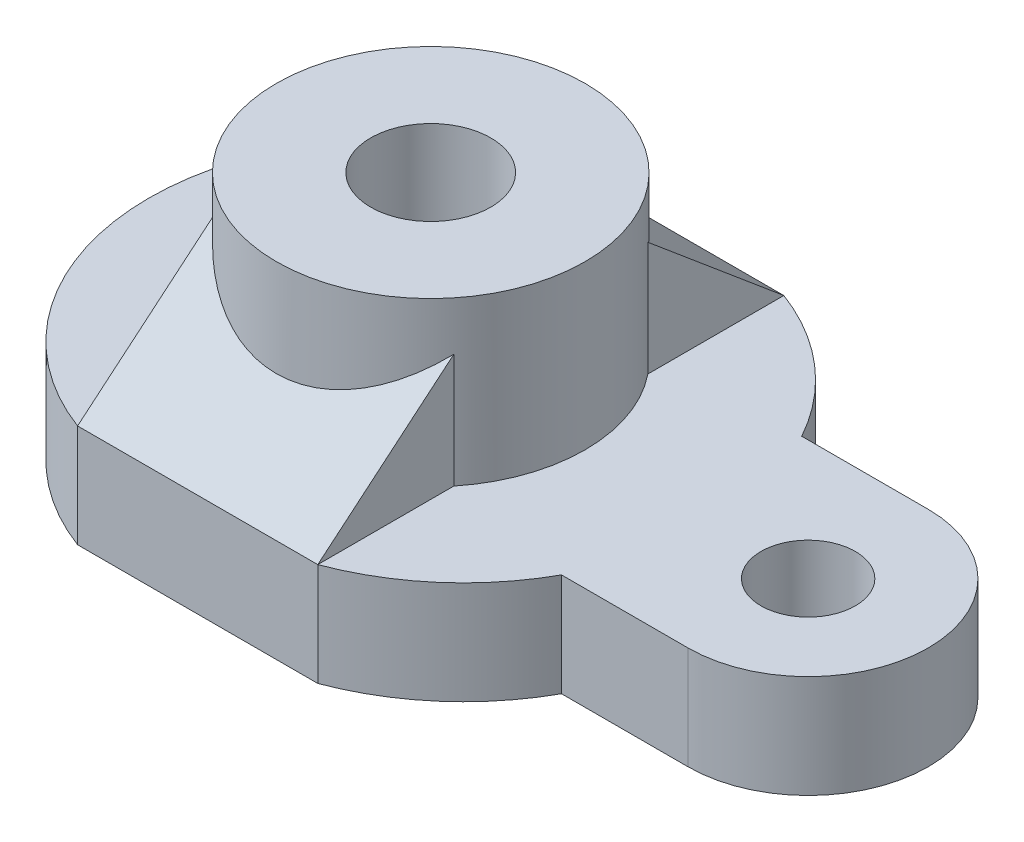
ISO-10303-21;
HEADER;
FILE_DESCRIPTION(('STEP AP214'),'2;1');
FILE_NAME('part.step','',(''),(''),'','','');
FILE_SCHEMA(('AUTOMOTIVE_DESIGN { 1 0 10303 214 1 1 1 1 }'));
ENDSEC;
DATA;
#1=APPLICATION_CONTEXT('core data for automotive mechanical design processes');
#2=APPLICATION_PROTOCOL_DEFINITION('international standard','automotive_design',2000,#1);
#3=PRODUCT_CONTEXT('',#1,'mechanical');
#4=PRODUCT('Part','Part','',(#3));
#5=PRODUCT_RELATED_PRODUCT_CATEGORY('part','',(#4));
#6=PRODUCT_DEFINITION_FORMATION('','',#4);
#7=PRODUCT_DEFINITION_CONTEXT('part definition',#1,'design');
#8=PRODUCT_DEFINITION('design','',#6,#7);
#9=PRODUCT_DEFINITION_SHAPE('','',#8);
#10=(LENGTH_UNIT() NAMED_UNIT(*) SI_UNIT(.MILLI.,.METRE.));
#11=(NAMED_UNIT(*) PLANE_ANGLE_UNIT() SI_UNIT($,.RADIAN.));
#12=(NAMED_UNIT(*) SI_UNIT($,.STERADIAN.) SOLID_ANGLE_UNIT());
#13=UNCERTAINTY_MEASURE_WITH_UNIT(LENGTH_MEASURE(1.E-05),#10,'distance_accuracy_value','');
#14=(GEOMETRIC_REPRESENTATION_CONTEXT(3) GLOBAL_UNCERTAINTY_ASSIGNED_CONTEXT((#13)) GLOBAL_UNIT_ASSIGNED_CONTEXT((#10,
#11,#12)) REPRESENTATION_CONTEXT('',''));
#15=CARTESIAN_POINT('',(0.,0.,0.));
#16=DIRECTION('',(0.,0.,1.));
#17=DIRECTION('',(1.,0.,0.));
#18=AXIS2_PLACEMENT_3D('',#15,#16,#17);
#19=CARTESIAN_POINT('',(-95.7034677287226,24.,0.));
#20=DIRECTION('',(0.,-1.,0.));
#21=DIRECTION('',(0.,0.,-1.));
#22=AXIS2_PLACEMENT_3D('',#19,#20,#21);
#23=PLANE('',#22);
#24=CARTESIAN_POINT('',(0.,24.,0.));
#25=DIRECTION('',(0.,1.,0.));
#26=DIRECTION('',(0.,0.,1.));
#27=AXIS2_PLACEMENT_3D('',#24,#25,#26);
#28=CIRCLE('',#27,11.);
#29=CARTESIAN_POINT('',(0.,24.,11.));
#30=VERTEX_POINT('',#29);
#31=EDGE_CURVE('E176',#30,#30,#28,.T.);
#32=ORIENTED_EDGE('',*,*,#31,.F.);
#33=EDGE_LOOP('',(#32));
#34=FACE_BOUND('',#33,.T.);
#35=DIRECTION('',(0.,0.,-1.));
#36=VECTOR('',#35,1.);
#37=CARTESIAN_POINT('',(-60.,24.,54.3327781156182));
#38=LINE('',#37,#36);
#39=CARTESIAN_POINT('',(-60.,24.,54.3327781156182));
#40=VERTEX_POINT('',#39);
#41=CARTESIAN_POINT('',(-60.,24.,22.6274169979695));
#42=VERTEX_POINT('',#41);
#43=EDGE_CURVE('E137',#40,#42,#38,.T.);
#44=ORIENTED_EDGE('',*,*,#43,.F.);
#45=CARTESIAN_POINT('',(-80.2965322712774,24.,0.));
#46=DIRECTION('',(0.,1.,0.));
#47=DIRECTION('',(0.,0.,-1.));
#48=AXIS2_PLACEMENT_3D('',#45,#46,#47);
#49=CIRCLE('',#48,58.);
#50=CARTESIAN_POINT('',(-29.5028318744762,24.,28.));
#51=VERTEX_POINT('',#50);
#52=EDGE_CURVE('E242',#40,#51,#49,.T.);
#53=ORIENTED_EDGE('',*,*,#52,.T.);
#54=DIRECTION('',(1.,0.,0.));
#55=VECTOR('',#54,1.);
#56=CARTESIAN_POINT('',(0.,24.,28.));
#57=LINE('',#56,#55);
#58=CARTESIAN_POINT('',(0.,24.,28.));
#59=VERTEX_POINT('',#58);
#60=EDGE_CURVE('E243',#51,#59,#57,.T.);
#61=ORIENTED_EDGE('',*,*,#60,.T.);
#62=CARTESIAN_POINT('',(0.,24.,0.));
#63=DIRECTION('',(0.,1.,0.));
#64=DIRECTION('',(0.,0.,1.));
#65=AXIS2_PLACEMENT_3D('',#62,#63,#64);
#66=CIRCLE('',#65,28.);
#67=CARTESIAN_POINT('',(0.,24.,-28.));
#68=VERTEX_POINT('',#67);
#69=EDGE_CURVE('E247',#59,#68,#66,.T.);
#70=ORIENTED_EDGE('',*,*,#69,.T.);
#71=DIRECTION('',(-1.,0.,0.));
#72=VECTOR('',#71,1.);
#73=CARTESIAN_POINT('',(0.,24.,-28.));
#74=LINE('',#73,#72);
#75=CARTESIAN_POINT('',(-29.5028318744762,24.,-28.));
#76=VERTEX_POINT('',#75);
#77=EDGE_CURVE('E155',#68,#76,#74,.T.);
#78=ORIENTED_EDGE('',*,*,#77,.T.);
#79=CARTESIAN_POINT('',(-80.2965322712774,24.,0.));
#80=DIRECTION('',(0.,1.,0.));
#81=DIRECTION('',(0.,0.,-1.));
#82=AXIS2_PLACEMENT_3D('',#79,#80,#81);
#83=CIRCLE('',#82,58.);
#84=CARTESIAN_POINT('',(-60.,24.,-54.3327781156181));
#85=VERTEX_POINT('',#84);
#86=EDGE_CURVE('E146',#76,#85,#83,.T.);
#87=ORIENTED_EDGE('',*,*,#86,.T.);
#88=CARTESIAN_POINT('',(-60.,24.,-22.6274169979695));
#89=VERTEX_POINT('',#88);
#90=EDGE_CURVE('E130',#89,#85,#38,.T.);
#91=ORIENTED_EDGE('',*,*,#90,.F.);
#92=CARTESIAN_POINT('',(-88.,24.,0.));
#93=DIRECTION('',(0.,1.,0.));
#94=DIRECTION('',(0.,0.,1.));
#95=AXIS2_PLACEMENT_3D('',#92,#93,#94);
#96=CIRCLE('',#95,36.);
#97=EDGE_CURVE('E212',#42,#89,#96,.T.);
#98=ORIENTED_EDGE('',*,*,#97,.F.);
#99=EDGE_LOOP('',(#44,#53,#61,#70,#78,#87,#91,#98));
#100=FACE_BOUND('',#99,.T.);
#101=ADVANCED_FACE('F39',(#34,#100),#23,.F.);
#102=CARTESIAN_POINT('',(-88.,62.,0.));
#103=DIRECTION('',(0.,-1.,0.));
#104=DIRECTION('',(0.,0.,-1.));
#105=AXIS2_PLACEMENT_3D('',#102,#103,#104);
#106=CYLINDRICAL_SURFACE('',#105,36.);
#107=CARTESIAN_POINT('',(-88.,62.,0.));
#108=DIRECTION('',(0.,1.,0.));
#109=DIRECTION('',(0.,0.,1.));
#110=AXIS2_PLACEMENT_3D('',#107,#108,#109);
#111=CIRCLE('',#110,36.);
#112=CARTESIAN_POINT('',(-88.,62.,36.));
#113=VERTEX_POINT('',#112);
#114=EDGE_CURVE('E232',#113,#113,#111,.T.);
#115=ORIENTED_EDGE('',*,*,#114,.F.);
#116=EDGE_LOOP('',(#115));
#117=FACE_BOUND('',#116,.T.);
#118=DIRECTION('',(0.,-1.,0.));
#119=VECTOR('',#118,1.);
#120=CARTESIAN_POINT('',(-60.,62.,-22.6274169979695));
#121=LINE('',#120,#119);
#122=CARTESIAN_POINT('',(-60.,50.6039568201611,-22.6274169979695));
#123=VERTEX_POINT('',#122);
#124=EDGE_CURVE('E11',#123,#89,#121,.T.);
#125=ORIENTED_EDGE('',*,*,#124,.F.);
#126=CARTESIAN_POINT('',(-88.,69.5906140776516,0.));
#127=DIRECTION('',(0.,-0.766044443118982,0.642787609686535));
#128=DIRECTION('',(0.,-0.642787609686535,-0.766044443118982));
#129=AXIS2_PLACEMENT_3D('',#126,#127,#128);
#130=ELLIPSE('',#129,46.9946624159618,36.);
#131=CARTESIAN_POINT('',(-116.,50.6039568201611,-22.6274169979695));
#132=VERTEX_POINT('',#131);
#133=EDGE_CURVE('E50',#132,#123,#130,.T.);
#134=ORIENTED_EDGE('',*,*,#133,.F.);
#135=DIRECTION('',(0.,-1.,0.));
#136=VECTOR('',#135,1.);
#137=CARTESIAN_POINT('',(-116.,62.,-22.6274169979695));
#138=LINE('',#137,#136);
#139=CARTESIAN_POINT('',(-116.,24.,-22.6274169979695));
#140=VERTEX_POINT('',#139);
#141=EDGE_CURVE('E217',#132,#140,#138,.T.);
#142=ORIENTED_EDGE('',*,*,#141,.T.);
#143=CARTESIAN_POINT('',(-116.,24.,22.6274169979695));
#144=VERTEX_POINT('',#143);
#145=EDGE_CURVE('E207',#140,#144,#96,.T.);
#146=ORIENTED_EDGE('',*,*,#145,.T.);
#147=DIRECTION('',(0.,-1.,0.));
#148=VECTOR('',#147,1.);
#149=CARTESIAN_POINT('',(-116.,62.,22.6274169979695));
#150=LINE('',#149,#148);
#151=CARTESIAN_POINT('',(-116.,50.6039568201612,22.6274169979695));
#152=VERTEX_POINT('',#151);
#153=EDGE_CURVE('E209',#144,#152,#150,.F.);
#154=ORIENTED_EDGE('',*,*,#153,.T.);
#155=CARTESIAN_POINT('',(-88.,69.5906140776517,0.));
#156=DIRECTION('',(0.,-0.766044443118982,-0.642787609686535));
#157=DIRECTION('',(0.,-0.642787609686535,0.766044443118982));
#158=AXIS2_PLACEMENT_3D('',#155,#156,#157);
#159=ELLIPSE('',#158,46.9946624159618,36.);
#160=CARTESIAN_POINT('',(-60.,50.6039568201612,22.6274169979695));
#161=VERTEX_POINT('',#160);
#162=EDGE_CURVE('E213',#161,#152,#159,.T.);
#163=ORIENTED_EDGE('',*,*,#162,.F.);
#164=DIRECTION('',(0.,-1.,0.));
#165=VECTOR('',#164,1.);
#166=CARTESIAN_POINT('',(-60.,62.,22.6274169979695));
#167=LINE('',#166,#165);
#168=EDGE_CURVE('E216',#42,#161,#167,.F.);
#169=ORIENTED_EDGE('',*,*,#168,.F.);
#170=ORIENTED_EDGE('',*,*,#97,.T.);
#171=EDGE_LOOP('',(#125,#134,#142,#146,#154,#163,#169,#170));
#172=FACE_BOUND('',#171,.T.);
#173=ADVANCED_FACE('F225',(#117,#172),#106,.T.);
#174=CARTESIAN_POINT('',(-95.7034677287226,24.,0.));
#175=DIRECTION('',(0.,1.,0.));
#176=DIRECTION('',(0.,0.,-1.));
#177=AXIS2_PLACEMENT_3D('',#174,#175,#176);
#178=CIRCLE('',#177,58.);
#179=CARTESIAN_POINT('',(-116.,24.,-54.3327781156181));
#180=VERTEX_POINT('',#179);
#181=CARTESIAN_POINT('',(-116.,24.,54.3327781156182));
#182=VERTEX_POINT('',#181);
#183=EDGE_CURVE('E192',#180,#182,#178,.T.);
#184=ORIENTED_EDGE('',*,*,#183,.T.);
#185=DIRECTION('',(0.,0.,-1.));
#186=VECTOR('',#185,1.);
#187=CARTESIAN_POINT('',(-116.,24.,54.3327781156182));
#188=LINE('',#187,#186);
#189=EDGE_CURVE('E227',#182,#144,#188,.T.);
#190=ORIENTED_EDGE('',*,*,#189,.T.);
#191=ORIENTED_EDGE('',*,*,#145,.F.);
#192=EDGE_CURVE('E62',#140,#180,#188,.T.);
#193=ORIENTED_EDGE('',*,*,#192,.T.);
#194=EDGE_LOOP('',(#184,#190,#191,#193));
#195=FACE_BOUND('',#194,.T.);
#196=ADVANCED_FACE('F226',(#195),#23,.F.);
#197=CARTESIAN_POINT('',(-95.7034677287226,0.,0.));
#198=DIRECTION('',(0.,-1.,0.));
#199=DIRECTION('',(0.,0.,-1.));
#200=AXIS2_PLACEMENT_3D('',#197,#198,#199);
#201=PLANE('',#200);
#202=CARTESIAN_POINT('',(-88.,0.,0.));
#203=DIRECTION('',(0.,-1.,0.));
#204=DIRECTION('',(0.,0.,-1.));
#205=AXIS2_PLACEMENT_3D('',#202,#203,#204);
#206=CIRCLE('',#205,14.);
#207=CARTESIAN_POINT('',(-88.,0.,-14.));
#208=VERTEX_POINT('',#207);
#209=EDGE_CURVE('E277',#208,#208,#206,.F.);
#210=ORIENTED_EDGE('',*,*,#209,.T.);
#211=EDGE_LOOP('',(#210));
#212=FACE_BOUND('',#211,.T.);
#213=CARTESIAN_POINT('',(-95.7034677287226,0.,0.));
#214=DIRECTION('',(0.,1.,0.));
#215=DIRECTION('',(0.,0.,-1.));
#216=AXIS2_PLACEMENT_3D('',#213,#214,#215);
#217=CIRCLE('',#216,58.);
#218=CARTESIAN_POINT('',(-116.,0.,-54.3327781156181));
#219=VERTEX_POINT('',#218);
#220=CARTESIAN_POINT('',(-116.,0.,54.3327781156182));
#221=VERTEX_POINT('',#220);
#222=EDGE_CURVE('E175',#219,#221,#217,.T.);
#223=ORIENTED_EDGE('',*,*,#222,.F.);
#224=DIRECTION('',(-1.,0.,0.));
#225=VECTOR('',#224,1.);
#226=CARTESIAN_POINT('',(-116.,0.,-54.3327781156181));
#227=LINE('',#226,#225);
#228=CARTESIAN_POINT('',(-60.,0.,-54.3327781156181));
#229=VERTEX_POINT('',#228);
#230=EDGE_CURVE('E190',#229,#219,#227,.T.);
#231=ORIENTED_EDGE('',*,*,#230,.F.);
#232=CARTESIAN_POINT('',(-80.2965322712774,0.,0.));
#233=DIRECTION('',(0.,1.,0.));
#234=DIRECTION('',(0.,0.,-1.));
#235=AXIS2_PLACEMENT_3D('',#232,#233,#234);
#236=CIRCLE('',#235,58.);
#237=CARTESIAN_POINT('',(-29.5028318744762,0.,-28.));
#238=VERTEX_POINT('',#237);
#239=EDGE_CURVE('E161',#238,#229,#236,.T.);
#240=ORIENTED_EDGE('',*,*,#239,.F.);
#241=DIRECTION('',(-1.,0.,0.));
#242=VECTOR('',#241,1.);
#243=CARTESIAN_POINT('',(0.,0.,-28.));
#244=LINE('',#243,#242);
#245=CARTESIAN_POINT('',(0.,0.,-28.));
#246=VERTEX_POINT('',#245);
#247=EDGE_CURVE('E187',#246,#238,#244,.T.);
#248=ORIENTED_EDGE('',*,*,#247,.F.);
#249=CARTESIAN_POINT('',(0.,0.,0.));
#250=DIRECTION('',(0.,1.,0.));
#251=DIRECTION('',(0.,0.,1.));
#252=AXIS2_PLACEMENT_3D('',#249,#250,#251);
#253=CIRCLE('',#252,28.);
#254=CARTESIAN_POINT('',(0.,0.,28.));
#255=VERTEX_POINT('',#254);
#256=EDGE_CURVE('E183',#255,#246,#253,.T.);
#257=ORIENTED_EDGE('',*,*,#256,.F.);
#258=DIRECTION('',(1.,0.,0.));
#259=VECTOR('',#258,1.);
#260=CARTESIAN_POINT('',(0.,0.,28.));
#261=LINE('',#260,#259);
#262=CARTESIAN_POINT('',(-29.5028318744762,0.,28.));
#263=VERTEX_POINT('',#262);
#264=EDGE_CURVE('E181',#263,#255,#261,.T.);
#265=ORIENTED_EDGE('',*,*,#264,.F.);
#266=CARTESIAN_POINT('',(-80.2965322712774,0.,0.));
#267=DIRECTION('',(0.,1.,0.));
#268=DIRECTION('',(0.,0.,-1.));
#269=AXIS2_PLACEMENT_3D('',#266,#267,#268);
#270=CIRCLE('',#269,58.);
#271=CARTESIAN_POINT('',(-60.,0.,54.3327781156182));
#272=VERTEX_POINT('',#271);
#273=EDGE_CURVE('E182',#272,#263,#270,.T.);
#274=ORIENTED_EDGE('',*,*,#273,.F.);
#275=DIRECTION('',(1.,0.,0.));
#276=VECTOR('',#275,1.);
#277=CARTESIAN_POINT('',(-116.,0.,54.3327781156182));
#278=LINE('',#277,#276);
#279=EDGE_CURVE('E180',#221,#272,#278,.T.);
#280=ORIENTED_EDGE('',*,*,#279,.F.);
#281=EDGE_LOOP('',(#223,#231,#240,#248,#257,#265,#274,#280));
#282=FACE_BOUND('',#281,.T.);
#283=CARTESIAN_POINT('',(0.,0.,0.));
#284=DIRECTION('',(0.,1.,0.));
#285=DIRECTION('',(0.,0.,1.));
#286=AXIS2_PLACEMENT_3D('',#283,#284,#285);
#287=CIRCLE('',#286,11.);
#288=CARTESIAN_POINT('',(0.,0.,11.));
#289=VERTEX_POINT('',#288);
#290=EDGE_CURVE('E233',#289,#289,#287,.T.);
#291=ORIENTED_EDGE('',*,*,#290,.T.);
#292=EDGE_LOOP('',(#291));
#293=FACE_BOUND('',#292,.T.);
#294=ADVANCED_FACE('F259',(#212,#282,#293),#201,.T.);
#295=CARTESIAN_POINT('',(-95.7034677287226,24.,0.));
#296=DIRECTION('',(0.,-1.,0.));
#297=DIRECTION('',(0.,0.,-1.));
#298=AXIS2_PLACEMENT_3D('',#295,#296,#297);
#299=CYLINDRICAL_SURFACE('',#298,58.);
#300=ORIENTED_EDGE('',*,*,#222,.T.);
#301=DIRECTION('',(0.,-1.,0.));
#302=VECTOR('',#301,1.);
#303=CARTESIAN_POINT('',(-116.,24.,54.3327781156182));
#304=LINE('',#303,#302);
#305=EDGE_CURVE('E206',#182,#221,#304,.T.);
#306=ORIENTED_EDGE('',*,*,#305,.F.);
#307=ORIENTED_EDGE('',*,*,#183,.F.);
#308=DIRECTION('',(0.,-1.,0.));
#309=VECTOR('',#308,1.);
#310=CARTESIAN_POINT('',(-116.,24.,-54.3327781156181));
#311=LINE('',#310,#309);
#312=EDGE_CURVE('E164',#180,#219,#311,.T.);
#313=ORIENTED_EDGE('',*,*,#312,.T.);
#314=EDGE_LOOP('',(#300,#306,#307,#313));
#315=FACE_BOUND('',#314,.T.);
#316=ADVANCED_FACE('F41',(#315),#299,.T.);
#317=CARTESIAN_POINT('',(-116.,24.,54.3327781156182));
#318=DIRECTION('',(0.,0.,-1.));
#319=DIRECTION('',(-1.,0.,0.));
#320=AXIS2_PLACEMENT_3D('',#317,#318,#319);
#321=PLANE('',#320);
#322=ORIENTED_EDGE('',*,*,#279,.T.);
#323=DIRECTION('',(0.,-1.,0.));
#324=VECTOR('',#323,1.);
#325=CARTESIAN_POINT('',(-60.,24.,54.3327781156182));
#326=LINE('',#325,#324);
#327=EDGE_CURVE('E201',#40,#272,#326,.T.);
#328=ORIENTED_EDGE('',*,*,#327,.F.);
#329=DIRECTION('',(1.,0.,0.));
#330=VECTOR('',#329,1.);
#331=CARTESIAN_POINT('',(-116.,24.,54.3327781156182));
#332=LINE('',#331,#330);
#333=EDGE_CURVE('E239',#182,#40,#332,.T.);
#334=ORIENTED_EDGE('',*,*,#333,.F.);
#335=ORIENTED_EDGE('',*,*,#305,.T.);
#336=EDGE_LOOP('',(#322,#328,#334,#335));
#337=FACE_BOUND('',#336,.T.);
#338=ADVANCED_FACE('F264',(#337),#321,.F.);
#339=CARTESIAN_POINT('',(-80.2965322712774,24.,0.));
#340=DIRECTION('',(0.,-1.,0.));
#341=DIRECTION('',(0.,0.,-1.));
#342=AXIS2_PLACEMENT_3D('',#339,#340,#341);
#343=CYLINDRICAL_SURFACE('',#342,58.);
#344=ORIENTED_EDGE('',*,*,#273,.T.);
#345=DIRECTION('',(0.,-1.,0.));
#346=VECTOR('',#345,1.);
#347=CARTESIAN_POINT('',(-29.5028318744762,24.,28.));
#348=LINE('',#347,#346);
#349=EDGE_CURVE('E199',#51,#263,#348,.T.);
#350=ORIENTED_EDGE('',*,*,#349,.F.);
#351=ORIENTED_EDGE('',*,*,#52,.F.);
#352=ORIENTED_EDGE('',*,*,#327,.T.);
#353=EDGE_LOOP('',(#344,#350,#351,#352));
#354=FACE_BOUND('',#353,.T.);
#355=ADVANCED_FACE('F335',(#354),#343,.T.);
#356=CARTESIAN_POINT('',(0.,24.,28.));
#357=DIRECTION('',(0.,0.,-1.));
#358=DIRECTION('',(-1.,0.,0.));
#359=AXIS2_PLACEMENT_3D('',#356,#357,#358);
#360=PLANE('',#359);
#361=ORIENTED_EDGE('',*,*,#264,.T.);
#362=DIRECTION('',(0.,-1.,0.));
#363=VECTOR('',#362,1.);
#364=CARTESIAN_POINT('',(0.,24.,28.));
#365=LINE('',#364,#363);
#366=EDGE_CURVE('E197',#59,#255,#365,.T.);
#367=ORIENTED_EDGE('',*,*,#366,.F.);
#368=ORIENTED_EDGE('',*,*,#60,.F.);
#369=ORIENTED_EDGE('',*,*,#349,.T.);
#370=EDGE_LOOP('',(#361,#367,#368,#369));
#371=FACE_BOUND('',#370,.T.);
#372=ADVANCED_FACE('F328',(#371),#360,.F.);
#373=CARTESIAN_POINT('',(0.,24.,0.));
#374=DIRECTION('',(0.,-1.,0.));
#375=DIRECTION('',(0.,0.,-1.));
#376=AXIS2_PLACEMENT_3D('',#373,#374,#375);
#377=CYLINDRICAL_SURFACE('',#376,28.);
#378=ORIENTED_EDGE('',*,*,#256,.T.);
#379=DIRECTION('',(0.,-1.,0.));
#380=VECTOR('',#379,1.);
#381=CARTESIAN_POINT('',(0.,24.,-28.));
#382=LINE('',#381,#380);
#383=EDGE_CURVE('E191',#68,#246,#382,.T.);
#384=ORIENTED_EDGE('',*,*,#383,.F.);
#385=ORIENTED_EDGE('',*,*,#69,.F.);
#386=ORIENTED_EDGE('',*,*,#366,.T.);
#387=EDGE_LOOP('',(#378,#384,#385,#386));
#388=FACE_BOUND('',#387,.T.);
#389=ADVANCED_FACE('F252',(#388),#377,.T.);
#390=CARTESIAN_POINT('',(0.,24.,-28.));
#391=DIRECTION('',(0.,0.,1.));
#392=DIRECTION('',(1.,0.,0.));
#393=AXIS2_PLACEMENT_3D('',#390,#391,#392);
#394=PLANE('',#393);
#395=ORIENTED_EDGE('',*,*,#247,.T.);
#396=DIRECTION('',(0.,-1.,0.));
#397=VECTOR('',#396,1.);
#398=CARTESIAN_POINT('',(-29.5028318744762,24.,-28.));
#399=LINE('',#398,#397);
#400=EDGE_CURVE('E163',#76,#238,#399,.T.);
#401=ORIENTED_EDGE('',*,*,#400,.F.);
#402=ORIENTED_EDGE('',*,*,#77,.F.);
#403=ORIENTED_EDGE('',*,*,#383,.T.);
#404=EDGE_LOOP('',(#395,#401,#402,#403));
#405=FACE_BOUND('',#404,.T.);
#406=ADVANCED_FACE('F258',(#405),#394,.F.);
#407=CARTESIAN_POINT('',(-80.2965322712774,24.,0.));
#408=DIRECTION('',(0.,-1.,0.));
#409=DIRECTION('',(0.,0.,-1.));
#410=AXIS2_PLACEMENT_3D('',#407,#408,#409);
#411=CYLINDRICAL_SURFACE('',#410,58.);
#412=ORIENTED_EDGE('',*,*,#239,.T.);
#413=DIRECTION('',(0.,-1.,0.));
#414=VECTOR('',#413,1.);
#415=CARTESIAN_POINT('',(-60.,24.,-54.3327781156181));
#416=LINE('',#415,#414);
#417=EDGE_CURVE('E158',#85,#229,#416,.T.);
#418=ORIENTED_EDGE('',*,*,#417,.F.);
#419=ORIENTED_EDGE('',*,*,#86,.F.);
#420=ORIENTED_EDGE('',*,*,#400,.T.);
#421=EDGE_LOOP('',(#412,#418,#419,#420));
#422=FACE_BOUND('',#421,.T.);
#423=ADVANCED_FACE('F157',(#422),#411,.T.);
#424=CARTESIAN_POINT('',(-116.,24.,-54.3327781156181));
#425=DIRECTION('',(0.,0.,1.));
#426=DIRECTION('',(1.,0.,0.));
#427=AXIS2_PLACEMENT_3D('',#424,#425,#426);
#428=PLANE('',#427);
#429=ORIENTED_EDGE('',*,*,#230,.T.);
#430=ORIENTED_EDGE('',*,*,#312,.F.);
#431=DIRECTION('',(-1.,0.,0.));
#432=VECTOR('',#431,1.);
#433=CARTESIAN_POINT('',(-116.,24.,-54.3327781156181));
#434=LINE('',#433,#432);
#435=EDGE_CURVE('E141',#85,#180,#434,.T.);
#436=ORIENTED_EDGE('',*,*,#435,.F.);
#437=ORIENTED_EDGE('',*,*,#417,.T.);
#438=EDGE_LOOP('',(#429,#430,#436,#437));
#439=FACE_BOUND('',#438,.T.);
#440=ADVANCED_FACE('F169',(#439),#428,.F.);
#441=CARTESIAN_POINT('',(0.,24.,0.));
#442=DIRECTION('',(0.,-1.,0.));
#443=DIRECTION('',(0.,0.,-1.));
#444=AXIS2_PLACEMENT_3D('',#441,#442,#443);
#445=CYLINDRICAL_SURFACE('',#444,11.);
#446=ORIENTED_EDGE('',*,*,#31,.T.);
#447=EDGE_LOOP('',(#446));
#448=FACE_BOUND('',#447,.T.);
#449=ORIENTED_EDGE('',*,*,#290,.F.);
#450=EDGE_LOOP('',(#449));
#451=FACE_BOUND('',#450,.T.);
#452=ADVANCED_FACE('F325',(#448,#451),#445,.F.);
#453=CARTESIAN_POINT('',(-88.,62.,0.));
#454=DIRECTION('',(0.,1.,0.));
#455=DIRECTION('',(0.,0.,1.));
#456=AXIS2_PLACEMENT_3D('',#453,#454,#455);
#457=PLANE('',#456);
#458=CARTESIAN_POINT('',(-88.,62.,0.));
#459=DIRECTION('',(0.,1.,0.));
#460=DIRECTION('',(0.,0.,1.));
#461=AXIS2_PLACEMENT_3D('',#458,#459,#460);
#462=CIRCLE('',#461,14.);
#463=CARTESIAN_POINT('',(-88.,62.,14.));
#464=VERTEX_POINT('',#463);
#465=EDGE_CURVE('E477',#464,#464,#462,.T.);
#466=ORIENTED_EDGE('',*,*,#465,.F.);
#467=EDGE_LOOP('',(#466));
#468=FACE_BOUND('',#467,.T.);
#469=ORIENTED_EDGE('',*,*,#114,.T.);
#470=EDGE_LOOP('',(#469));
#471=FACE_BOUND('',#470,.T.);
#472=ADVANCED_FACE('F296',(#468,#471),#457,.T.);
#473=CARTESIAN_POINT('',(-116.,0.,0.));
#474=DIRECTION('',(-1.,0.,0.));
#475=DIRECTION('',(0.,0.,1.));
#476=AXIS2_PLACEMENT_3D('',#473,#474,#475);
#477=PLANE('',#476);
#478=ORIENTED_EDGE('',*,*,#153,.F.);
#479=ORIENTED_EDGE('',*,*,#189,.F.);
#480=DIRECTION('',(0.,-0.642787609686535,0.766044443118982));
#481=VECTOR('',#480,1.);
#482=CARTESIAN_POINT('',(-116.,24.,54.3327781156182));
#483=LINE('',#482,#481);
#484=EDGE_CURVE('E53',#152,#182,#483,.T.);
#485=ORIENTED_EDGE('',*,*,#484,.F.);
#486=EDGE_LOOP('',(#478,#479,#485));
#487=FACE_BOUND('',#486,.T.);
#488=ADVANCED_FACE('F285',(#487),#477,.T.);
#489=CARTESIAN_POINT('',(-60.,0.,0.));
#490=DIRECTION('',(-1.,0.,0.));
#491=DIRECTION('',(0.,0.,1.));
#492=AXIS2_PLACEMENT_3D('',#489,#490,#491);
#493=PLANE('',#492);
#494=ORIENTED_EDGE('',*,*,#43,.T.);
#495=ORIENTED_EDGE('',*,*,#168,.T.);
#496=DIRECTION('',(0.,-0.642787609686535,0.766044443118982));
#497=VECTOR('',#496,1.);
#498=CARTESIAN_POINT('',(-60.,24.,54.3327781156182));
#499=LINE('',#498,#497);
#500=EDGE_CURVE('E144',#161,#40,#499,.T.);
#501=ORIENTED_EDGE('',*,*,#500,.T.);
#502=EDGE_LOOP('',(#494,#495,#501));
#503=FACE_BOUND('',#502,.T.);
#504=ADVANCED_FACE('F291',(#503),#493,.F.);
#505=CARTESIAN_POINT('',(-60.,24.,54.3327781156182));
#506=DIRECTION('',(0.,-0.766044443118982,-0.642787609686535));
#507=DIRECTION('',(0.,0.642787609686535,-0.766044443118982));
#508=AXIS2_PLACEMENT_3D('',#505,#506,#507);
#509=PLANE('',#508);
#510=ORIENTED_EDGE('',*,*,#500,.F.);
#511=ORIENTED_EDGE('',*,*,#162,.T.);
#512=ORIENTED_EDGE('',*,*,#484,.T.);
#513=ORIENTED_EDGE('',*,*,#333,.T.);
#514=EDGE_LOOP('',(#510,#511,#512,#513));
#515=FACE_BOUND('',#514,.T.);
#516=ADVANCED_FACE('F269',(#515),#509,.F.);
#517=DIRECTION('',(0.,0.642787609686535,0.766044443118982));
#518=VECTOR('',#517,1.);
#519=CARTESIAN_POINT('',(-60.,58.4587439801252,-13.2664461810193));
#520=LINE('',#519,#518);
#521=EDGE_CURVE('E128',#85,#123,#520,.T.);
#522=ORIENTED_EDGE('',*,*,#521,.T.);
#523=ORIENTED_EDGE('',*,*,#124,.T.);
#524=ORIENTED_EDGE('',*,*,#90,.T.);
#525=EDGE_LOOP('',(#522,#523,#524));
#526=FACE_BOUND('',#525,.T.);
#527=ADVANCED_FACE('F129',(#526),#493,.F.);
#528=ORIENTED_EDGE('',*,*,#141,.F.);
#529=DIRECTION('',(0.,0.642787609686535,0.766044443118982));
#530=VECTOR('',#529,1.);
#531=CARTESIAN_POINT('',(-116.,58.4587439801252,-13.2664461810193));
#532=LINE('',#531,#530);
#533=EDGE_CURVE('E281',#180,#132,#532,.T.);
#534=ORIENTED_EDGE('',*,*,#533,.F.);
#535=ORIENTED_EDGE('',*,*,#192,.F.);
#536=EDGE_LOOP('',(#528,#534,#535));
#537=FACE_BOUND('',#536,.T.);
#538=ADVANCED_FACE('F282',(#537),#477,.T.);
#539=CARTESIAN_POINT('',(-60.,58.4587439801252,-13.2664461810193));
#540=DIRECTION('',(0.,-0.766044443118982,0.642787609686535));
#541=DIRECTION('',(0.,-0.642787609686535,-0.766044443118982));
#542=AXIS2_PLACEMENT_3D('',#539,#540,#541);
#543=PLANE('',#542);
#544=ORIENTED_EDGE('',*,*,#533,.T.);
#545=ORIENTED_EDGE('',*,*,#133,.T.);
#546=ORIENTED_EDGE('',*,*,#521,.F.);
#547=ORIENTED_EDGE('',*,*,#435,.T.);
#548=EDGE_LOOP('',(#544,#545,#546,#547));
#549=FACE_BOUND('',#548,.T.);
#550=ADVANCED_FACE('F143',(#549),#543,.F.);
#551=CARTESIAN_POINT('',(-88.,-0.001000000000001,0.));
#552=DIRECTION('',(0.,1.,0.));
#553=DIRECTION('',(0.,0.,1.));
#554=AXIS2_PLACEMENT_3D('',#551,#552,#553);
#555=CYLINDRICAL_SURFACE('',#554,14.);
#556=ORIENTED_EDGE('',*,*,#209,.F.);
#557=EDGE_LOOP('',(#556));
#558=FACE_BOUND('',#557,.T.);
#559=ORIENTED_EDGE('',*,*,#465,.T.);
#560=EDGE_LOOP('',(#559));
#561=FACE_BOUND('',#560,.T.);
#562=ADVANCED_FACE('F288',(#558,#561),#555,.F.);
#563=CLOSED_SHELL('',(#101,#173,#196,#294,#316,#338,#355,#372,#389,#406,#423,#440,#452,#472,
#488,#504,#516,#527,#538,#550,#562));
#564=MANIFOLD_SOLID_BREP('B2',#563);
#565=ADVANCED_BREP_SHAPE_REPRESENTATION('',(#18,#564),#14);
#566=SHAPE_DEFINITION_REPRESENTATION(#9,#565);
ENDSEC;
END-ISO-10303-21;
